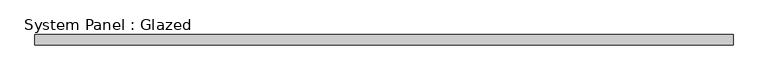
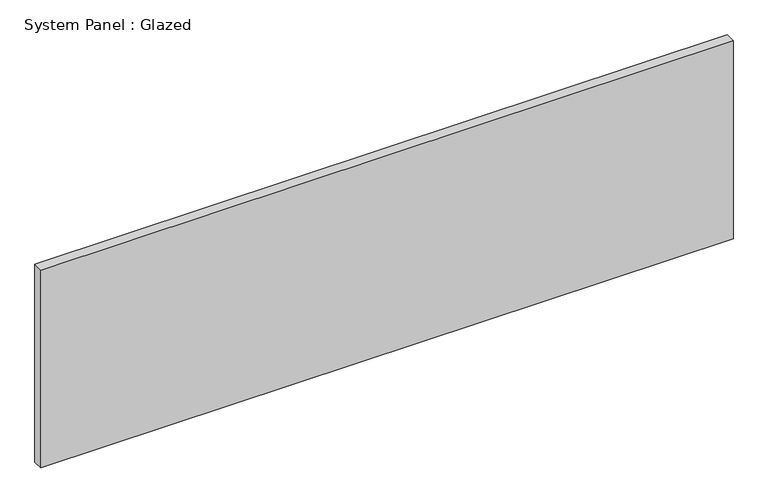
"""IFC4 building model written with IfcOpenShell, lengths in millimetres: plate geometry, System Panel : Glazed."""

from ifc_helpers import new_model, si_unit, origin, origin_with_axes, place, context, project, spatial, polyline, outline, extrude, source, transform, mapped, element, save


def system_panel_glazed_c29578c4(model_context):
    return source(origin(), model_context, "Body", "SweptSolid", [
        extrude(outline(polyline([(850.9, 19.05), (-850.9, 19.05), (-850.9, 44.45), (850.9, 44.45), (850.9, 19.05)])), origin_with_axes(), (0.0, 0.0, 1.0), 514.35),
    ])


if __name__ == "__main__":
    model = new_model("IFC4")
    model_context = context("Model", 3, world=origin())
    ifc_project = project(units=[si_unit("LENGTHUNIT", "METRE", prefix="MILLI")], contexts=[model_context])
    site = spatial("IfcSite", under=ifc_project)
    building = spatial("IfcBuilding", under=site)
    placement = place(None, origin())
    system_panel_glazed_shape = system_panel_glazed_c29578c4(model_context)
    element("IfcPlate", 1, ObjectType="System Panel : Glazed", at=placement, inside=building, context=model_context, shape_type="MappedRepresentation", body=[
        mapped(system_panel_glazed_shape, transform((0.0, 0.0, 0.0), x_axis=(1.0, 0.0, 0.0), y_axis=(0.0, 1.0, 0.0), z_axis=(0.0, 0.0, 1.0))),
    ])
    save(model, "model.ifc")

# Revit data of these elements
# Type "System Panel : Glazed"
#   Construction Type Id = "GSP4R"
#   Analytic Construction = "1/8 in Pilkington single glazing"
#   Visual Light Transmittance = 0.9
#   Solar Heat Gain Coefficient = 0.86
#   Heat Transfer Coefficient (U) = 1.18115 BTU/(h·ft²·°F)
# Element 1 (IfcPlate, "System Panel : Glazed")
#   Materials on its faces: "Glass"
# Materials
#   "Glass": class "Glass", colour RGB 0 128 192, transparency 0.75, Description = "Soda Lime Glass", Cost = 0
